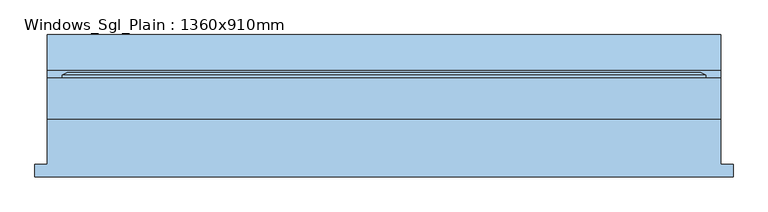
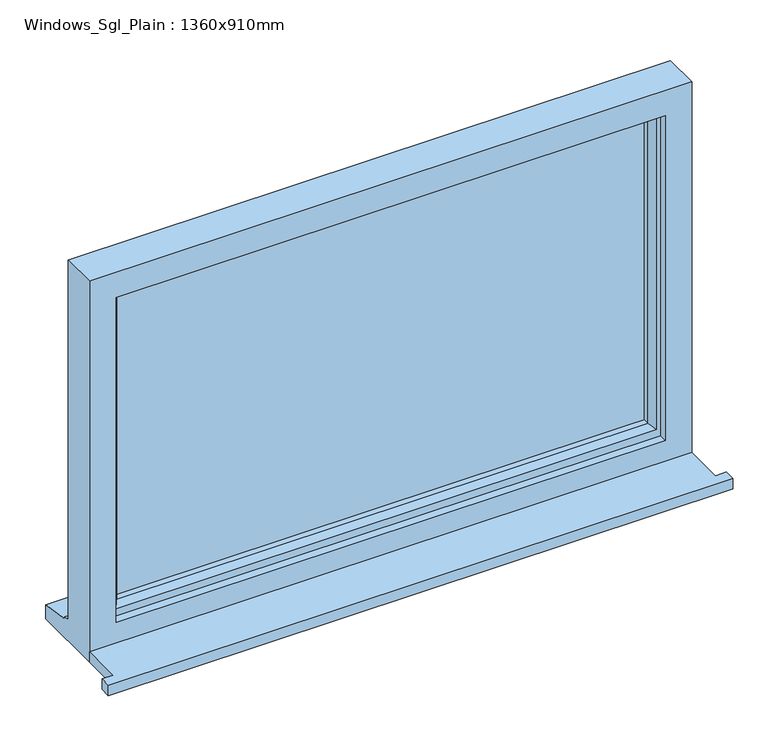
"""IFC4 building model written with IfcOpenShell, lengths in millimetres: window geometry, Windows_Sgl_Plain : 1360x910mm."""

from ifc_helpers import new_model, si_unit, frame, origin, place, context, project, spatial, polyline, outline, extrude, faceted_brep, source, transform, mapped, element, save


def windows_sgl_plain_1360x910mm_f5b307ae(model_context):
    return source(origin(), model_context, "Body", "SolidModel", [
        extrude(outline(polyline([(-705.0, -129.0434322), (-705.0, -104.0434322), (-680.0, -104.0434322), (-680.0, -12.0434322), (680.0, -12.0434322), (680.0, -104.0434322), (705.0, -104.0434322), (705.0, -129.0434322), (-705.0, -129.0434322)])), frame((0.0, 0.0, 1200.0), z_axis=(0.0, 0.0, 1.0), x_axis=(1.0, 0.0, 0.0)), (0.0, 0.0, 1.0), 25.0),
        faceted_brep([(-680.0, -12.0434322, 1200.0), (680.0, -12.0434322, 1200.0), (680.0, -12.0434322, 2110.0), (-680.0, -12.0434322, 2110.0), (-620.0, -12.0434322, 2050.0), (620.0, -12.0434322, 2050.0), (620.0, -12.0434322, 1275.0), (-620.0, -12.0434322, 1275.0), (-680.0, 70.9565678, 2110.0), (-680.0, 70.9565678, 1251.0), (-680.0, 85.9565678, 1249.68767), (-680.0, 85.9565678, 1244.7449676), (-680.0, 158.4565678, 1233.8088847), (-680.0, 158.4565678, 1200.0), (680.0, 70.9565678, 2110.0), (680.0, 70.9565678, 1251.0), (-640.0, 70.9565678, 2070.0), (-640.0, 70.9565678, 1263.0), (640.0, 70.9565678, 1263.0), (640.0, 70.9565678, 2070.0), (-640.0, 5.9565678, 2070.0), (-640.0, 5.9565678, 1263.0), (640.0, 5.9565678, 2070.0), (640.0, 5.9565678, 1263.0), (-620.0, 5.9565678, 2050.0), (-620.0, 5.9565678, 1275.0), (620.0, 5.9565678, 1275.0), (620.0, 5.9565678, 2050.0), (680.0, 158.4565678, 1200.0), (680.0, 158.4565678, 1233.8088847), (680.0, 85.9565678, 1244.7449676), (680.0, 85.9565678, 1249.68767)], [[[0, 1, 2, 3], [4, 5, 6, 7]], [[0, 3, 8, 9, 10, 11, 12, 13]], [[9, 8, 14, 15], [16, 17, 18, 19]], [[17, 16, 20, 21]], [[20, 22, 23, 21], [24, 25, 26, 27]], [[24, 4, 7, 25]], [[3, 2, 14, 8]], [[16, 19, 22, 20]], [[5, 4, 24, 27]], [[15, 14, 2, 1, 28, 29, 30, 31]], [[19, 18, 23, 22]], [[5, 27, 26, 6]], [[28, 1, 0, 13]], [[29, 28, 13, 12]], [[30, 29, 12, 11]], [[31, 30, 11, 10]], [[15, 31, 10, 9]], [[21, 23, 18, 17]], [[7, 6, 26, 25]]]),
        extrude(outline(polyline([(610.0, 34.9565678), (-610.0, 34.9565678), (-610.0, 58.9565678), (610.0, 58.9565678), (610.0, 34.9565678)])), frame((0.0, 0.0, 1293.0), z_axis=(0.0, 0.0, 1.0), x_axis=(1.0, 0.0, 0.0)), (0.0, 0.0, 1.0), 747.0),
        faceted_brep([(-650.0, 70.9565678, 2080.0), (-650.0, 76.7300705, 2080.0), (-650.0, 76.7300705, 1253.0), (-650.0, 70.9565678, 1253.0), (-640.0, 5.9565678, 2070.0), (-640.0, 70.9565678, 2070.0), (-640.0, 70.9565678, 1263.0), (-640.0, 5.9565678, 1263.0), (-600.0, 20.4494677, 2030.0), (-610.1480377, 5.9565678, 2040.1480377), (-610.1480377, 5.9565678, 1292.8519623), (-600.0, 20.4494677, 1303.0), (-600.0, 34.9565678, 2030.0), (-600.0, 34.9565678, 1303.0), (-610.0, 58.9565678, 2040.0), (-610.0, 34.9565678, 2040.0), (-610.0, 34.9565678, 1293.0), (-610.0, 58.9565678, 1293.0), (-600.0, 76.7300705, 2030.0), (-600.0, 58.9565678, 2030.0), (-600.0, 58.9565678, 1303.0), (-600.0, 76.7300705, 1303.0), (-617.4457548, 82.5035732, 2047.4457548), (-617.4457548, 82.5035732, 1285.5542452), (-639.2153903, 82.5035732, 2069.2153903), (-639.2153903, 82.5035732, 1263.7846097), (650.0, 76.7300705, 1253.0), (650.0, 70.9565678, 1253.0), (640.0, 70.9565678, 1263.0), (640.0, 5.9565678, 1263.0), (610.1480377, 5.9565678, 1292.8519623), (600.0, 20.4494677, 1303.0), (600.0, 34.9565678, 1303.0), (610.0, 34.9565678, 1293.0), (610.0, 58.9565678, 1293.0), (600.0, 58.9565678, 1303.0), (600.0, 76.7300705, 1303.0), (617.4457548, 82.5035732, 1285.5542452), (639.2153903, 82.5035732, 1263.7846097), (650.0, 76.7300705, 2080.0), (650.0, 70.9565678, 2080.0), (640.0, 70.9565678, 2070.0), (640.0, 5.9565678, 2070.0), (610.1480377, 5.9565678, 2040.1480377), (600.0, 20.4494677, 2030.0), (600.0, 34.9565678, 2030.0), (610.0, 34.9565678, 2040.0), (610.0, 58.9565678, 2040.0), (600.0, 58.9565678, 2030.0), (600.0, 76.7300705, 2030.0), (617.4457548, 82.5035732, 2047.4457548), (639.2153903, 82.5035732, 2069.2153903)], [[[0, 1, 2, 3]], [[4, 5, 6, 7]], [[8, 9, 10, 11]], [[12, 8, 11, 13]], [[14, 15, 16, 17]], [[18, 19, 20, 21]], [[22, 18, 21, 23]], [[1, 24, 25, 2]], [[3, 2, 26, 27]], [[7, 6, 28, 29]], [[11, 10, 30, 31]], [[13, 11, 31, 32]], [[17, 16, 33, 34]], [[21, 20, 35, 36]], [[23, 21, 36, 37]], [[2, 25, 38, 26]], [[27, 26, 39, 40]], [[29, 28, 41, 42]], [[31, 30, 43, 44]], [[32, 31, 44, 45]], [[34, 33, 46, 47]], [[36, 35, 48, 49]], [[37, 36, 49, 50]], [[26, 38, 51, 39]], [[40, 39, 1, 0]], [[3, 27, 40, 0], [5, 41, 28, 6]], [[42, 41, 5, 4]], [[7, 29, 42, 4], [9, 43, 30, 10]], [[44, 43, 9, 8]], [[45, 44, 8, 12]], [[15, 46, 33, 16], [13, 32, 45, 12]], [[47, 46, 15, 14]], [[17, 34, 47, 14], [19, 48, 35, 20]], [[49, 48, 19, 18]], [[50, 49, 18, 22]], [[24, 51, 38, 25], [23, 37, 50, 22]], [[39, 51, 24, 1]]]),
    ])


if __name__ == "__main__":
    model = new_model("IFC4")
    model_context = context("Model", 3, world=origin())
    ifc_project = project(units=[si_unit("LENGTHUNIT", "METRE", prefix="MILLI")], contexts=[model_context])
    site = spatial("IfcSite", under=ifc_project)
    building = spatial("IfcBuilding", under=site)
    placement = place(None, origin())
    windows_sgl_plain_1360x910mm_shape = windows_sgl_plain_1360x910mm_f5b307ae(model_context)
    element("IfcWindow", 1, ObjectType="Windows_Sgl_Plain : 1360x910mm", at=placement, inside=building, context=model_context, shape_type="MappedRepresentation", body=[
        mapped(windows_sgl_plain_1360x910mm_shape, transform((0.0, 0.0, 0.0), x_axis=(1.0, 0.0, 0.0), y_axis=(0.0, 1.0, 0.0), z_axis=(0.0, 0.0, 1.0))),
    ])
    save(model, "model.ifc")

# Revit data of these elements
# Type "Windows_Sgl_Plain : 1360x910mm"
#   Type Mark = "46"
#   Operation = "SinglePanel"
#   Construction Type Id = "SGL"
#   Manufacturer = "Revit"
#   Keynote = "L10"
#   Analytic Construction = "Large single-glazed windows"
#   Wrap Layers (Ext) from Ext = 102.5 mm
#   Wrap Layers (Int) from Ext = 177.5 mm
#   Window Board Projection = 25 mm
#   Window Board Extension = 25 mm
#   Visual Light Transmittance = 0.9
#   Solar Heat Gain Coefficient = 0.86
#   Rough Width = 1360 mm
#   Rough Height = 910 mm
#   Height = 910 mm
#   Width = 1360 mm
#   Heat Transfer Coefficient (U) = 5.5617 W/(m²·K)
#   Glazing Thickness = 24 mm
#   FrameOffset - External = 50 mm
#   Frame Depth = 65 mm
#   Default Head Height = 2110 mm
#   Cill Depth = 87.5 mm
#   Cavity Closer Width = 50 mm
#   Cavity Closer Offset from Ext = 102.5 mm
#   Cavity Closer Depth = 85 mm
#   Define Thermal Properties by = 1
#   Vis - Cavity Closers = yes
#   Define Thermal Properties by = 1
#   Material Trim = Window Frame
#   Material Glass = Glass
#   Material Frame = Window Frame
#   Wall Closure = (empty or 0)
# Element 1 (IfcWindow, "Windows_Sgl_Plain : 1360x910mm")
#   Materials on its faces: "Window Frame", "Glass"
# Materials
#   "Window Frame": colour RGB 249 249 249, transparency 0, Keynote = "L10", Cost = 0
#   "Glass": class "Glass", colour RGB 0 128 192, transparency 0.9, Description = "Soda Lime Glass", Cost = 0
